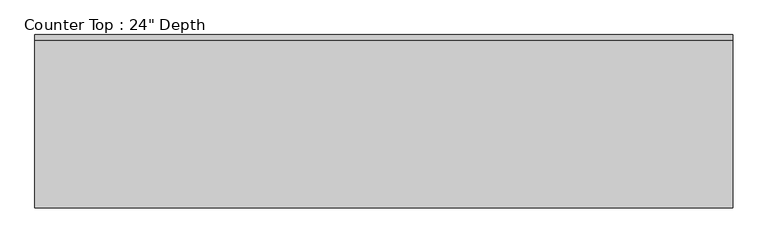
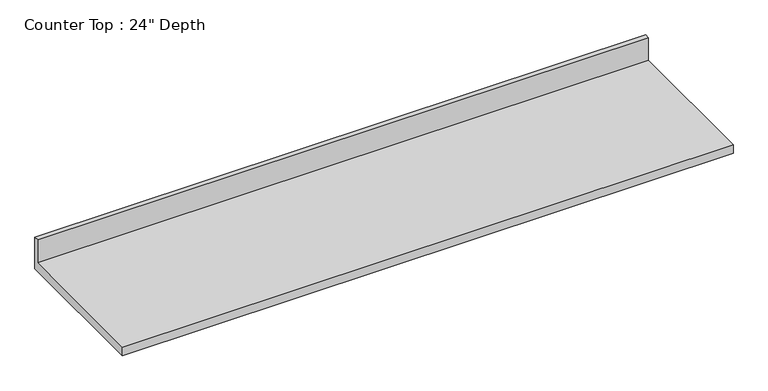
"""IFC4 building model written with IfcOpenShell, lengths in millimetres: furniture geometry."""

from ifc_helpers import new_model, si_unit, frame, origin, place, context, project, spatial, polyline, outline, extrude, source, transform, mapped, element, save


def furniture_1a836c3b(model_context):
    return source(origin(), model_context, "Body", "SweptSolid", [
        extrude(outline(polyline([(0.0, 1016.0), (0.0, 876.3), (-635.0, 876.3), (-635.0, 914.4), (-19.05, 914.4), (-19.05, 1016.0), (0.0, 1016.0)])), frame((-1200.4622951, 0.0, 0.0), z_axis=(1.0, 0.0, 0.0), x_axis=(0.0, 1.0, 0.0)), (0.0, 0.0, 1.0), 2556.9724958),
    ])


if __name__ == "__main__":
    model = new_model("IFC4")
    model_context = context("Model", 3, world=origin())
    ifc_project = project(units=[si_unit("LENGTHUNIT", "METRE", prefix="MILLI")], contexts=[model_context])
    site = spatial("IfcSite", under=ifc_project)
    building = spatial("IfcBuilding", under=site)
    placement = place(None, origin())
    furniture_shape = furniture_1a836c3b(model_context)
    element("IfcFurniture", 1, ObjectType="Counter Top : 24\" Depth", at=placement, inside=building, context=model_context, shape_type="MappedRepresentation", body=[
        mapped(furniture_shape, transform((0.0, 0.0, 0.0), x_axis=(1.0, 0.0, 0.0), y_axis=(0.0, 1.0, 0.0), z_axis=(0.0, 0.0, 1.0))),
    ])
    save(model, "model.ifc")

# Revit data of these elements
# Type "Counter Top : 24\" Depth"
#   Assembly Code = "C1030400"
#   Counter Thickness = 0' - 1 1/2"
#   Depth = 2' - 1"
#   Height = 3' - 0"
#   Length [instance default] = 8' - 0"
#   Counter Top Material = none
#   Default Elevation = 0
# Element 1 (IfcFurniture, "Counter Top : 24\" Depth")
#   Length = 8' - 4.66821"
#   Materials on its faces: "Counter Top"
# Materials
#   "Counter Top": class "Wood", colour RGB 226 177 128, transparency 0
